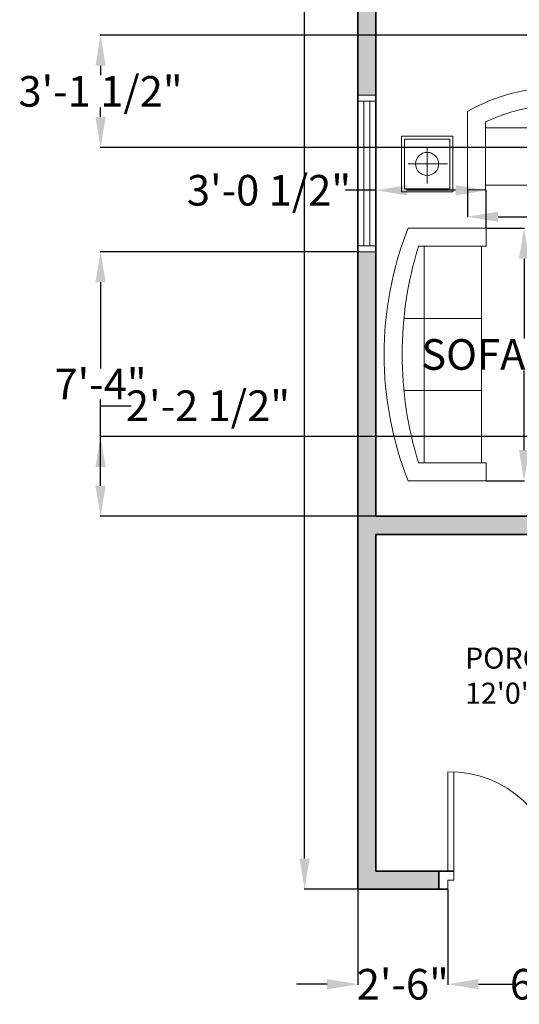
# Model space of a CAD drawing. Units: inches. Extents: x 1294 to 2470, y 659 to 1389.
# Tile 1 of 4: x 1294 to 1460, y 704 to 1031. Entities that reach past the tile are written whole.
import ezdxf

# ---------------------------------------------------------------- set-up
doc = ezdxf.new("R2010")
doc.units = ezdxf.units.IN
doc.header["$MEASUREMENT"] = 0
for name, color, linetype, lineweight in [('A-ANNO-DIMS', 2, 'Continuous', 18), ('A-AREA-IDEN', 7, 'Continuous', 20), ('A-DOOR', 3, 'Continuous', 18), ('A-FURN', 8, 'Continuous', 18), ('A-GLAZ', 4, 'Continuous', 18), ('A-WALL', 7, 'Continuous', 35), ('A-WALL-PATT', 252, 'Continuous', 13)]:
    doc.layers.add(name, color=color, linetype=linetype, lineweight=lineweight)
doc.styles.get("Standard").update_dxf_attribs({"font": 'arial.ttf'})
doc.dimstyles.get("Standard").update_dxf_attribs({"dimtxt": 10.18, "dimasz": 10.18, "dimexe": 0.18, "dimexo": 0.0625, "dimgap": 0.09, "dimtad": 0, "dimtih": 1, "dimtoh": 1, "dimdec": 0, "dimzin": 0, "dimdsep": 46, "dimlunit": 3, "dimtxsty": 'Standard', "dimcen": 0.09, "dimadec": 0, "dimazin": 0, "dimtfac": 1, "dimtdec": 0, "dimtofl": 0, "dimtmove": 0, "dimatfit": 3, "dimfxl": 1, "dimtolj": 1, "dimtzin": 0, "dimarcsym": 0})

# ---------------------------------------------------------------- blocks, each defined once
blk = doc.blocks.new('Sofa - Roundback 7 ft.')
for p, q in [((-12.00002, -32.4421), (-12.00003, -6.5971)), ((11.99997, -32.4421), (11.99998, -6.5971)), ((-36.000027, -34), (-36.000027, -11.4696)), ((35.99998, -34), (35.99998, -11.4696)), ((-35.999844, -13.3819), (35.9998, -13.3819)), ((-36.000027, -32.4421), (35.99998, -32.4421))]:
    blk.add_line(p, q)
for points in [[(-36.000027, -34), (-42.000027, -34), (-42.000027, -8)], [(41.99998, -8), (41.99998, -34), (35.99998, -34)]]:
    blk.add_lwpolyline(points)
for centre, radius, start, end in [((0, -114.25), 114.25, 68.43141, 111.5686), ((-0.00001, -127.1968), 121.1968, 72.72033, 107.2797)]:
    blk.add_arc(centre, radius, start, end)
blk = doc.blocks.new('Sofa - Roundback Loveseat 5 ft.')
for p, q in [((0, -32.44198), (0, -5.99998)), ((-24, -33.99998), (-24, -11.46958)), ((24.00004, -33.99998), (24.00004, -11.46958)), ((-23.9998, -13.38178), (23.99986, -13.38178)), ((-24, -32.44198), (24.00004, -32.44198))]:
    blk.add_line(p, q)
for points in [[(-24, -33.99998), (-30, -33.99998), (-30, -7.99998)], [(30.00004, -7.99998), (30.00004, -33.99998), (24.00004, -33.99998)]]:
    blk.add_lwpolyline(points)
for centre, radius, start, end in [((0, -60.24998), 60.24998, 60.13715, 119.8628), ((0, -61.38438), 55.38444, 64.32083, 115.6792)]:
    blk.add_arc(centre, radius, start, end)
blk = doc.blocks.new('*D6')
at = {"layer": 'A-ANNO-DIMS', "color": 0, "lineweight": -2, "transparency": 16777216}
for p, q in [((1406.6, 1341.78), (1388.79, 1341.78)), ((1388.97, 1331.6), (1388.97, 1047.07)), ((1388.97, 751.96), (1388.97, 1036.5)), ((1406.6, 741.78), (1388.79, 741.78))]:
    blk.add_line(p, q, dxfattribs=at)
at = {"layer": 'A-ANNO-DIMS', "color": 0, "transparency": 16777216}
for points in [[(1387.28, 1331.6), (1390.67, 1331.6), (1388.97, 1341.78)], [(1387.28, 751.96), (1390.67, 751.96), (1388.97, 741.78)]]:
    blk.add_solid(points, dxfattribs=at)
at = {"layer": 'Defpoints', "color": 0, "transparency": 16777216}
for p in [(1406.66, 1341.78), (1388.97, 741.78), (1406.66, 741.78)]:
    blk.add_point(p, dxfattribs=at)
at = {"layer": 'A-ANNO-DIMS', "color": 0, "transparency": 16777216, "insert": (1388.97, 1041.78), "char_height": 10.18, "attachment_point": 5}
blk.add_mtext("\\A1;50'", dxfattribs=at)
blk = doc.blocks.new('WIN-48')
for p, q in [((0, 6), (0, 0)), ((2, 6), (2, 0)), ((50, 4), (2, 4)), ((50, 6), (50, 0)), ((52, 6), (52, 0)), ((50, 2), (2, 2))]:
    blk.add_line(p, q)
blk = doc.blocks.new('*D28')
at = {"layer": 'A-ANNO-DIMS', "color": 0, "lineweight": -2, "transparency": 16777216}
for p, q in [((1449.5, 961.6), (1462.22, 961.6)), ((1462.04, 951.42), (1462.04, 924.95)), ((1462.04, 887.78), (1462.04, 914.24)), ((1449.5, 877.6), (1462.22, 877.6))]:
    blk.add_line(p, q, dxfattribs=at)
at = {"layer": 'A-ANNO-DIMS', "color": 0, "transparency": 16777216}
for points in [[(1460.34, 951.42), (1463.74, 951.42), (1462.04, 961.6)], [(1460.34, 887.78), (1463.74, 887.78), (1462.04, 877.6)]]:
    blk.add_solid(points, dxfattribs=at)
at = {"layer": 'Defpoints', "color": 0, "transparency": 16777216}
for p in [(1449.44, 961.6), (1462.04, 961.6), (1449.44, 877.6)]:
    blk.add_point(p, dxfattribs=at)
at = {"layer": 'A-ANNO-DIMS', "color": 0, "transparency": 16777216, "insert": (1462.04, 919.6), "char_height": 10.18, "attachment_point": 5}
blk.add_mtext('\\A1;SOFA 7\'-0"', dxfattribs=at)
blk = doc.blocks.new('*D29')
at = {"layer": 'A-ANNO-DIMS', "color": 0, "lineweight": -2, "transparency": 16777216}
for p, q in [((1412.77, 974.2), (1402.59, 974.2)), ((1412.77, 961.66), (1412.77, 974.38)), ((1439.26, 974.2), (1422.95, 974.2)), ((1449.44, 961.66), (1449.44, 974.38))]:
    blk.add_line(p, q, dxfattribs=at)
at = {"layer": 'A-ANNO-DIMS', "color": 0, "transparency": 16777216}
for points in [[(1422.95, 975.89), (1422.95, 972.5), (1412.77, 974.2)], [(1439.26, 975.89), (1439.26, 972.5), (1449.44, 974.2)]]:
    blk.add_solid(points, dxfattribs=at)
at = {"layer": 'Defpoints', "color": 0, "transparency": 16777216}
for p in [(1412.77, 974.2), (1412.77, 961.6), (1449.44, 961.6)]:
    blk.add_point(p, dxfattribs=at)
at = {"layer": 'A-ANNO-DIMS', "color": 0, "transparency": 16777216, "insert": (1377.12, 974.2), "char_height": 10.18, "attachment_point": 5}
blk.add_mtext('\\A1;3\'-0 1/2"', dxfattribs=at)
blk = doc.blocks.new('*D30')
at = {"layer": 'A-ANNO-DIMS', "color": 0, "lineweight": -2, "transparency": 16777216}
for p, q in [((1443.19, 974.33), (1443.19, 965.21)), ((1503.19, 974.33), (1503.19, 965.21)), ((1453.37, 965.39), (1493.01, 965.39)), ((1503.19, 965.39), (1513.37, 965.39))]:
    blk.add_line(p, q, dxfattribs=at)
at = {"layer": 'A-ANNO-DIMS', "color": 0, "transparency": 16777216}
for points in [[(1453.37, 967.09), (1453.37, 963.7), (1443.19, 965.39)], [(1493.01, 967.09), (1493.01, 963.7), (1503.19, 965.39)]]:
    blk.add_solid(points, dxfattribs=at)
at = {"layer": 'Defpoints', "color": 0, "transparency": 16777216}
for p in [(1443.19, 974.39), (1503.19, 974.39), (1503.19, 965.39)]:
    blk.add_point(p, dxfattribs=at)
at = {"layer": 'A-ANNO-DIMS', "color": 0, "transparency": 16777216, "insert": (1566.29, 965.39), "char_height": 10.18, "attachment_point": 5}
blk.add_mtext('\\A1;LOVESEAT 5\'-0"', dxfattribs=at)
blk = doc.blocks.new('*D34')
at = {"layer": 'A-ANNO-DIMS', "color": 0, "lineweight": -2, "transparency": 16777216}
for p, q in [((1436.66, 741.72), (1436.66, 710)), ((1508.66, 741.72), (1508.66, 710)), ((1446.84, 710.18), (1459.01, 710.18)), ((1498.48, 710.18), (1486.31, 710.18))]:
    blk.add_line(p, q, dxfattribs=at)
at = {"layer": 'A-ANNO-DIMS', "color": 0, "transparency": 16777216}
for points in [[(1446.84, 711.88), (1446.84, 708.49), (1436.66, 710.18)], [(1498.48, 711.88), (1498.48, 708.49), (1508.66, 710.18)]]:
    blk.add_solid(points, dxfattribs=at)
at = {"layer": 'Defpoints', "color": 0, "transparency": 16777216}
for p in [(1436.66, 741.78), (1508.66, 741.78), (1508.66, 710.18)]:
    blk.add_point(p, dxfattribs=at)
at = {"layer": 'A-ANNO-DIMS', "color": 0, "transparency": 16777216, "insert": (1472.66, 710.18), "char_height": 10.18, "attachment_point": 5}
blk.add_mtext('\\A1;6\'-0"', dxfattribs=at)
blk = doc.blocks.new('*D35')
at = {"layer": 'A-ANNO-DIMS', "color": 0, "lineweight": -2, "transparency": 16777216}
for p, q in [((1406.66, 741.72), (1406.66, 710)), ((1436.66, 741.72), (1436.66, 710)), ((1396.48, 710.18), (1386.3, 710.18)), ((1446.84, 710.18), (1457.02, 710.18))]:
    blk.add_line(p, q, dxfattribs=at)
at = {"layer": 'A-ANNO-DIMS', "color": 0, "transparency": 16777216}
for points in [[(1396.48, 711.88), (1396.48, 708.49), (1406.66, 710.18)], [(1446.84, 711.88), (1446.84, 708.49), (1436.66, 710.18)]]:
    blk.add_solid(points, dxfattribs=at)
at = {"layer": 'Defpoints', "color": 0, "transparency": 16777216}
for p in [(1406.66, 741.78), (1436.66, 741.78), (1436.66, 710.18)]:
    blk.add_point(p, dxfattribs=at)
at = {"layer": 'A-ANNO-DIMS', "color": 0, "transparency": 16777216, "insert": (1421.66, 710.18), "char_height": 10.18, "attachment_point": 5}
blk.add_mtext('\\A1;2\'-6"', dxfattribs=at)
blk = doc.blocks.new('*D46')
at = {"layer": 'A-ANNO-DIMS', "color": 0, "lineweight": -2, "transparency": 16777216}
for p, q in [((1406.6, 953.78), (1320.88, 953.78)), ((1321.06, 943.6), (1321.06, 914.96)), ((1321.06, 875.96), (1321.06, 904.6)), ((1412.6, 865.78), (1320.88, 865.78))]:
    blk.add_line(p, q, dxfattribs=at)
at = {"layer": 'A-ANNO-DIMS', "color": 0, "transparency": 16777216}
for points in [[(1319.37, 943.6), (1322.76, 943.6), (1321.06, 953.78)], [(1319.37, 875.96), (1322.76, 875.96), (1321.06, 865.78)]]:
    blk.add_solid(points, dxfattribs=at)
at = {"layer": 'Defpoints', "color": 0, "transparency": 16777216}
for p in [(1321.06, 953.78), (1406.66, 953.78), (1412.66, 865.78)]:
    blk.add_point(p, dxfattribs=at)
at = {"layer": 'A-ANNO-DIMS', "color": 0, "transparency": 16777216, "insert": (1321.06, 909.78), "char_height": 10.18, "attachment_point": 5}
blk.add_mtext('\\A1;7\'-4"', dxfattribs=at)
blk = doc.blocks.new('*D47')
at = {"layer": 'A-ANNO-DIMS', "color": 0, "lineweight": -2, "transparency": 16777216}
for p, q in [((1532.6, 1025.78), (1320.88, 1025.78)), ((1321.06, 1015.6), (1321.06, 1012.46)), ((1321.06, 998.59), (1321.06, 1001.74)), ((1538.6, 988.41), (1320.88, 988.41))]:
    blk.add_line(p, q, dxfattribs=at)
at = {"layer": 'A-ANNO-DIMS', "color": 0, "transparency": 16777216}
for points in [[(1319.37, 1015.6), (1322.76, 1015.6), (1321.06, 1025.78)], [(1319.37, 998.59), (1322.76, 998.59), (1321.06, 988.41)]]:
    blk.add_solid(points, dxfattribs=at)
at = {"layer": 'Defpoints', "color": 0, "transparency": 16777216}
for p in [(1321.06, 1025.78), (1532.66, 1025.78), (1538.66, 988.41)]:
    blk.add_point(p, dxfattribs=at)
at = {"layer": 'A-ANNO-DIMS', "color": 0, "transparency": 16777216, "insert": (1321.06, 1007.1), "char_height": 10.18, "attachment_point": 5}
blk.add_mtext('\\A1;3\'-1 1/2"', dxfattribs=at)
blk = doc.blocks.new('*D52')
at = {"layer": 'A-ANNO-DIMS', "color": 0, "lineweight": -2, "transparency": 16777216}
for p, q in [((1321.06, 892.37), (1321.06, 902.55)), ((1321.06, 902.55), (1331.24, 902.55)), ((1538.6, 892.37), (1320.88, 892.37)), ((1321.06, 875.96), (1321.06, 882.19)), ((1538.6, 865.78), (1320.88, 865.78))]:
    blk.add_line(p, q, dxfattribs=at)
at = {"layer": 'A-ANNO-DIMS', "color": 0, "transparency": 16777216}
for points in [[(1319.37, 882.19), (1322.76, 882.19), (1321.06, 892.37)], [(1319.37, 875.96), (1322.76, 875.96), (1321.06, 865.78)]]:
    blk.add_solid(points, dxfattribs=at)
at = {"layer": 'Defpoints', "color": 0, "transparency": 16777216}
for p in [(1321.06, 892.37), (1538.66, 892.37), (1538.66, 865.78)]:
    blk.add_point(p, dxfattribs=at)
at = {"layer": 'A-ANNO-DIMS', "color": 0, "transparency": 16777216, "insert": (1356.81, 902.55), "char_height": 10.18, "attachment_point": 5}
blk.add_mtext('\\A1;2\'-2 1/2"', dxfattribs=at)

msp = doc.modelspace()

# ---------------------------------------------------------------- hatches: boundary and pattern name
at = {"layer": 'A-WALL-PATT'}
h = msp.add_hatch(color=256, dxfattribs=at)
h.dxf.hatch_style = 1
h.paths.add_polyline_path([(1412.66, 1335.78), (1446.66, 1335.78), (1446.66, 1341.78), (1406.66, 1341.78), (1406.66, 1197.78), (1412.66, 1197.78), (1412.66, 1213.78), (1480.66, 1213.78), (1480.66, 1186.78), (1481.11, 1186.78, -0.021978), (1483.66, 1186.78), (1486.66, 1186.78), (1486.66, 1213.78), (1493.66, 1213.78), (1493.66, 1216.78, -0.014283), (1493.66, 1218.78), (1493.66, 1219.78), (1412.66, 1219.78)])
h.paths.add_polyline_path([(1563.66, 1341.78), (1498.66, 1341.78), (1498.66, 1335.78), (1532.66, 1335.78), (1532.66, 1219.78), (1532.66, 1213.78), (1538.66, 1213.78), (1538.66, 1219.78), (1538.66, 1335.78), (1563.66, 1335.78)])
h.paths.add_polyline_path([(1646.66, 1341.78), (1615.66, 1341.78), (1615.66, 1335.78), (1640.66, 1335.78), (1640.66, 1219.78), (1622.13, 1219.78), (1622.13, 1216.78, -0.017236), (1622.13, 1214.78), (1622.13, 1213.78), (1640.66, 1213.78), (1640.66, 1197.78), (1646.66, 1197.78)])
h.paths.add_polyline_path([(1646.66, 1169.78), (1640.66, 1169.78), (1640.66, 1153.78), (1577.66, 1153.78), (1577.66, 1150.78, -0.014283), (1577.66, 1148.78), (1577.66, 1147.78), (1640.66, 1147.78), (1640.66, 1115.78), (1646.66, 1115.78)])
h.paths.add_polyline_path([(1589.13, 1213.78), (1583.13, 1213.78), (1583.13, 1153.78), (1589.13, 1153.78)])
h.paths.add_polyline_path([(1538.66, 1147.78), (1538.66, 1153.78), (1532.66, 1153.78), (1532.66, 1025.78), (1538.66, 1025.78), (1640.66, 1025.78), (1640.66, 971.78), (1646.66, 971.78), (1646.66, 1063.78), (1640.66, 1063.78), (1640.66, 1031.78), (1538.66, 1031.78)])
h.paths.add_polyline_path([(1486.66, 1153.78), (1480.66, 1153.78), (1412.66, 1153.78), (1412.66, 1169.78), (1406.66, 1169.78), (1406.66, 1137.78), (1412.66, 1137.78), (1412.66, 1147.78), (1460.66, 1147.78), (1466.66, 1147.78), (1486.66, 1147.78)])
h.paths.add_polyline_path([(1466.66, 1099.78), (1460.66, 1099.78), (1412.66, 1099.78), (1412.66, 1109.78), (1406.66, 1109.78), (1406.66, 1005.78), (1412.66, 1005.78), (1412.66, 1093.78), (1466.66, 1093.78)])
h.paths.add_polyline_path([(1412.66, 953.78), (1406.66, 953.78), (1406.66, 741.78), (1433.66, 741.78), (1433.66, 747.78), (1412.66, 747.78), (1412.66, 859.78), (1493.66, 859.78), (1493.66, 862.78, -0.014283), (1493.66, 864.78), (1493.66, 865.78), (1412.66, 865.78)])
h.paths.add_polyline_path([(1538.66, 988.41), (1532.66, 988.41), (1532.66, 865.78), (1532.66, 859.78), (1538.66, 859.78), (1640.66, 859.78), (1640.66, 747.78), (1538.66, 747.78), (1532.66, 747.78), (1511.66, 747.78), (1511.66, 741.78), (1646.66, 741.78), (1646.66, 919.78), (1640.66, 919.78), (1640.66, 865.78), (1538.66, 865.78)])

# ---------------------------------------------------------------- linework, layer by layer
at = {"layer": 'A-DOOR'}
for p, q in [((1436.66, 747.78), (1436.66, 780.78)), ((1438.66, 744.78), (1438.66, 780.78)), ((1436.66, 744.78), (1436.66, 741.78)), ((1438.66, 744.78), (1436.66, 744.78))]:
    msp.add_line(p, q, dxfattribs=at)
msp.add_arc((1437.66, 745.78), 35.01, 1.6366, 91.6366, dxfattribs=at)
at = {"layer": 'A-FURN'}
for p, q in [((1429.76, 982.96), (1429.76, 988.57)), ((1429.76, 988.57), (1429.76, 976.47)), ((1429.76, 982.96), (1423.42, 982.96)), ((1423.42, 982.96), (1436.49, 982.96))]:
    msp.add_line(p, q, dxfattribs=at)
for points in [[(1421.18, 992.22), (1421.18, 992.22), (1438.33, 992.22), (1438.33, 992.22), (1438.33, 973.69), (1438.33, 973.69), (1421.18, 973.69), (1421.18, 973.69)], [(1422.18, 991.22), (1437.33, 991.22), (1437.33, 974.69), (1422.18, 974.69)]]:
    msp.add_lwpolyline(points, close=True, dxfattribs=at)
msp.add_circle((1429.76, 982.96), 3.84, dxfattribs=at)
at = {"layer": 'A-WALL'}
for p, q in [((1406.66, 741.78), (1406.66, 1341.78)), ((1412.66, 865.78), (1412.66, 1093.78)), ((1412.66, 865.78), (1493.7, 865.78)), ((1412.66, 747.78), (1412.66, 859.78)), ((1412.66, 859.78), (1493.66, 859.78)), ((1438.66, 747.78), (1412.66, 747.78)), ((1433.66, 747.78), (1433.66, 741.78)), ((1436.66, 741.78), (1406.66, 741.78))]:
    msp.add_line(p, q, dxfattribs=at)

# ---------------------------------------------------------------- block references
at = {"layer": 'A-FURN'}
msp.add_blockref('Sofa - Roundback Loveseat 5 ft.', (1473.19, 1008.39), dxfattribs=at)
at = {"layer": 'A-FURN', "rotation": 90}
msp.add_blockref('Sofa - Roundback 7 ft.', (1415.44, 919.6), dxfattribs=at)
at = {"layer": 'A-GLAZ', "rotation": 269.9999999999989}
msp.add_blockref('WIN-48', (1406.66, 1005.78), dxfattribs=at)

# ---------------------------------------------------------------- texts
at = {"layer": 'A-AREA-IDEN', "insert": (1442.37, 822.13), "char_height": 7, "attachment_point": 1}
msp.add_mtext_dynamic_manual_height_columns('PORCH\\P12\'0"X10\'0"', width=68.5815, gutter_width=1, heights=[0], dxfattribs=at)

# ---------------------------------------------------------------- dimensions: what is measured, and where the dimension line sits
at = {"layer": 'A-ANNO-DIMS'}
for base, p1, p2, angle, override, picture, middle in [((1388.97, 741.78), (1406.66, 1341.78), (1406.66, 741.78), 90, {"dimclrd": 0, "dimclre": 0, "dimclrt": 0}, '*D6', (1388.97, 1041.78)), ((1321.06, 1025.78), (1538.66, 988.41), (1532.66, 1025.78), 90, {"dimdec": 1, "dimlfac": 1, "dimrnd": 0, "dimzin": 1, "dimdsep": 46, "dimlunit": 4, "dimfrac": 2}, '*D47', (1321.06, 1007.1)), ((1412.77, 974.2), (1449.44, 961.6), (1412.77, 961.6), 180, {"dimdec": 1, "dimlfac": 1, "dimrnd": 0, "dimzin": 1, "dimdsep": 46, "dimlunit": 4, "dimfrac": 2}, '*D29', (1377.12, 974.2)), ((1321.06, 953.78), (1412.66, 865.78), (1406.66, 953.78), 90, {"dimdec": 1, "dimlfac": 1, "dimrnd": 0, "dimzin": 1, "dimdsep": 46, "dimlunit": 4, "dimfrac": 2}, '*D46', (1321.06, 909.78)), ((1321.06, 892.37), (1538.66, 865.78), (1538.66, 892.37), 90, {"dimdec": 1, "dimlfac": 1, "dimrnd": 0, "dimzin": 1, "dimdsep": 46, "dimlunit": 4, "dimfrac": 2}, '*D52', (1356.81, 902.55))]:
    dim = msp.add_linear_dim(base=base, p1=p1, p2=p2, angle=angle, dimstyle='Standard', override=override, dxfattribs=at)
    dim.commit()
    dim.dimension.update_dxf_attribs({"geometry": picture, "text_midpoint": middle})
dim = msp.add_linear_dim(base=(1503.19, 965.39), p1=(1443.19, 974.39), p2=(1503.19, 974.39), text='LOVESEAT <>', dimstyle='Standard', override={"dimdec": 1, "dimlfac": 1, "dimrnd": 0, "dimzin": 1, "dimdsep": 46, "dimlunit": 4, "dimfrac": 2}, dxfattribs=at)
dim.commit()
dim.dimension.update_dxf_attribs({"geometry": '*D30', "text_midpoint": (1566.29, 965.39)})
dim = msp.add_linear_dim(base=(1462.04, 961.6), p1=(1449.44, 877.6), p2=(1449.44, 961.6), angle=90, text='SOFA <>', dimstyle='Standard', override={"dimdec": 1, "dimlfac": 1, "dimrnd": 0, "dimzin": 1, "dimdsep": 46, "dimlunit": 4, "dimfrac": 2}, dxfattribs=at)
dim.commit()
dim.dimension.update_dxf_attribs({"geometry": '*D28', "text_midpoint": (1462.04, 919.6)})
for base, p1, p2, picture, middle in [((1436.66, 710.18), (1406.66, 741.78), (1436.66, 741.78), '*D35', (1421.66, 710.18)), ((1508.66, 710.18), (1436.66, 741.78), (1508.66, 741.78), '*D34', (1472.66, 710.18))]:
    dim = msp.add_linear_dim(base=base, p1=p1, p2=p2, dimstyle='Standard', override={"dimdec": 1, "dimlfac": 1, "dimrnd": 0, "dimzin": 1, "dimdsep": 46, "dimlunit": 4, "dimfrac": 2}, dxfattribs=at)
    dim.commit()
    dim.dimension.update_dxf_attribs({"geometry": picture, "text_midpoint": middle})

doc.saveas('drawing.dxf')
